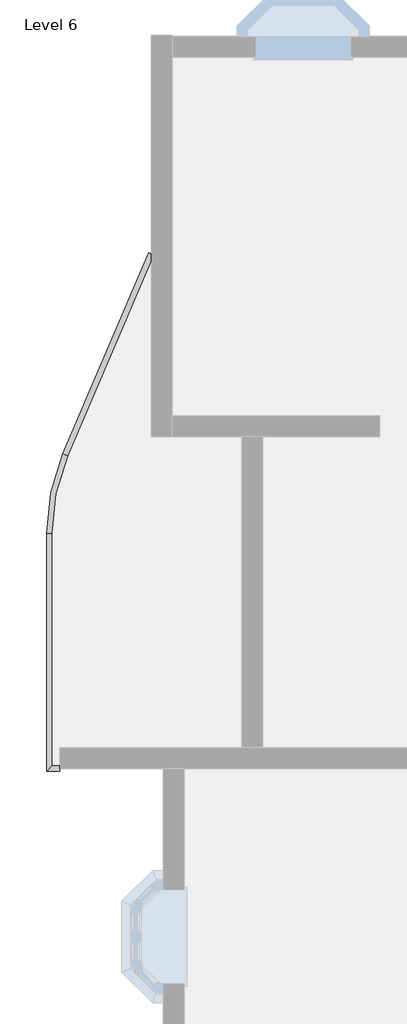
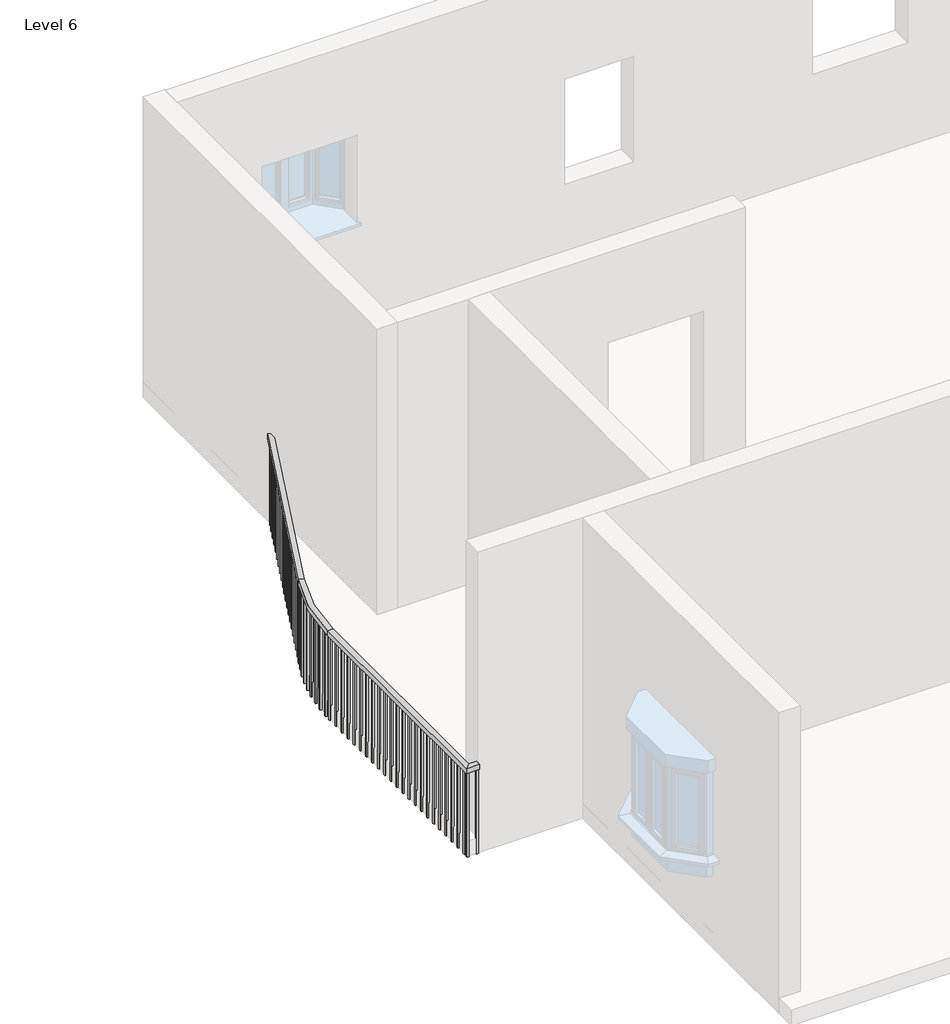
# One storey, part 7 of 14: 1 railing.
"""IFC4 building model written with IfcOpenShell, lengths in millimetres."""

from ifc_helpers import new_model, si_unit, frame, origin, place, context, project, spatial, polyline, circle_curve, outline, extrude, element, save
from ifc_brep_helpers import plane_surface, cylinder_surface, revolved_surface, advanced_brep

model = new_model("IFC4")

# Units and contexts
model_context = context("Model", 3, world=origin())
ifc_project = project(units=[si_unit("LENGTHUNIT", "METRE", prefix="MILLI")], contexts=[model_context])

# Site, building, storey
site = spatial("IfcSite", under=ifc_project)
building = spatial("IfcBuilding", under=site)
storey = spatial("IfcBuildingStorey", under=building, Name="Level 6", Elevation=15240.0)

# Railing
placement = place(None, origin())
element("IfcRailing", 1, ObjectType="Handrail - Rectangular", at=placement, inside=storey, context=model_context, shape_type="SolidModel", body=[
    advanced_brep(
    [(-12381.4379579, -2441.2590879, 16154.4), (-12381.4379579, -2441.2590879, 16103.6), (-12428.1364721, -2421.2618688, 16103.6), (-12428.1364721, -2421.2618688, 16154.4), (-13216.1814979, -4390.5942894, 16154.4), (-13216.1814979, -4390.5942894, 16103.6), (-13262.8800121, -4370.5970703, 16103.6), (-13262.8800121, -4370.5970703, 16154.4), (-13369.987215, -5140.4900045, 16103.6), (-13369.987215, -5140.4900045, 16154.4), (-13420.787215, -5140.4900045, 16103.6), (-13420.787215, -5140.4900045, 16154.4), (-13369.987215, -7396.5416506, 16154.4), (-13369.987215, -7396.5416506, 16103.6), (-13420.787215, -7447.3416506, 16103.6), (-13420.787215, -7447.3416506, 16154.4), (-13293.787215, -7396.5416506, 16154.4), (-13293.787215, -7447.3416506, 16154.4), (-13293.787215, -7447.3416506, 16103.6), (-13293.787215, -7396.5416506, 16103.6)],
    [
        (0, 1),
        (1, 2),
        (2, 3),
        (3, 0),
        (0, 4),
        (4, 5),
        (5, 1),
        (5, 6),
        (6, 2),
        (6, 7),
        (7, 3),
        (7, 4),
        (8, 5, circle_curve(frame((-11464.987215, -5140.4900045, 16103.6), z_axis=(0.0, 0.0, -1.0), x_axis=(-0.9192620907623801, 0.39364604467361003, 0.0)), 1905.0)),
        (4, 9, circle_curve(frame((-11464.987215, -5140.4900045, 16154.4), z_axis=(0.0, 0.0, 1.0), x_axis=(-0.9192620907623801, 0.39364604467361003, 0.0)), 1905.0)),
        (9, 8),
        (10, 6, circle_curve(frame((-11464.987215, -5140.4900045, 16103.6), z_axis=(0.0, 0.0, -1.0), x_axis=(-0.9192620907623801, 0.39364604467361003, 0.0)), 1955.8)),
        (8, 10),
        (11, 7, circle_curve(frame((-11464.987215, -5140.4900045, 16154.4), z_axis=(0.0, 0.0, -1.0), x_axis=(-0.9192620907623801, 0.39364604467361003, 0.0)), 1955.8)),
        (10, 11),
        (11, 9),
        (9, 12),
        (12, 13),
        (13, 8),
        (13, 14),
        (14, 10),
        (14, 15),
        (15, 11),
        (15, 12),
        (16, 17),
        (17, 18),
        (18, 19),
        (19, 16),
        (12, 16),
        (19, 13),
        (18, 14),
        (17, 15),
    ],
    [
        plane_surface(frame((-12404.787215, -2431.2604783, 16154.4), z_axis=(0.39364604467361003, 0.9192620907623801, 0.0), x_axis=(0.9192620907623801, -0.39364604467361003, 0.0))),
        plane_surface(frame((-12381.4379579, -2441.2590879, 16154.4), z_axis=(0.91926209076238, -0.39364604467361014, 0.0), x_axis=(-0.39364604467361014, -0.91926209076238, 0.0))),
        plane_surface(frame((-12381.4379579, -2441.2590879, 16103.6), z_axis=(0.0, 0.0, -1.0), x_axis=(-0.39364604467361014, -0.91926209076238, 0.0))),
        plane_surface(frame((-12428.1364721, -2421.2618688, 16103.6), z_axis=(-0.91926209076238, 0.39364604467361014, 0.0), x_axis=(-0.39364604467361014, -0.91926209076238, 0.0))),
        plane_surface(frame((-12428.1364721, -2421.2618688, 16154.4), z_axis=(0.0, 0.0, 1.0), x_axis=(-0.39364604467361014, -0.91926209076238, 0.0))),
        revolved_surface(polyline([(-13216.181497902333, -4390.594289396773, 16154.4), (-13216.181497902333, -4390.594289396773, 16103.6)]), (-11464.987215, -5140.4900045, 16154.4), (0.0, 0.0, 1.0)),
        plane_surface(frame((-11464.987215, -5140.4900045, 16103.6), z_axis=(0.0, 0.0, -1.0000000000000002), x_axis=(-0.9192620907623801, 0.39364604467361003, 0.0))),
        cylinder_surface(frame((-11464.987215, -5140.4900045, 16154.4), z_axis=(0.0, 0.0, 1.0), x_axis=(-0.9192620907623801, 0.39364604467361003, 0.0)), 1955.8),
        plane_surface(frame((-11464.987215, -5140.4900045, 16154.4), z_axis=(0.0, 0.0, 1.0000000000000002), x_axis=(-0.9192620907623801, 0.39364604467361003, 0.0))),
        plane_surface(frame((-13369.987215, -5140.4900045, 16154.4), z_axis=(1.0, 0.0, 0.0), x_axis=(0.0, -1.0, 0.0))),
        plane_surface(frame((-13369.987215, -5140.4900045, 16103.6), z_axis=(0.0, 0.0, -1.0), x_axis=(0.0, -1.0, 0.0))),
        plane_surface(frame((-13420.787215, -5140.4900045, 16103.6), z_axis=(-1.0, 0.0, 0.0), x_axis=(0.0, -1.0, 0.0))),
        plane_surface(frame((-13420.787215, -5140.4900045, 16154.4), z_axis=(0.0, 0.0, 1.0), x_axis=(0.0, -1.0, 0.0))),
        plane_surface(frame((-13293.787215, -7421.9416506, 16154.4), z_axis=(1.0, 0.0, 0.0), x_axis=(0.0, 1.0, 0.0))),
        plane_surface(frame((-13369.987215, -7396.5416506, 16154.4), z_axis=(0.0, 1.0, 0.0), x_axis=(1.0, 0.0, 0.0))),
        plane_surface(frame((-13369.987215, -7396.5416506, 16103.6), z_axis=(0.0, 0.0, -1.0), x_axis=(1.0, 0.0, 0.0))),
        plane_surface(frame((-13420.787215, -7447.3416506, 16103.6), z_axis=(0.0, -1.0, 0.0), x_axis=(1.0, 0.0, 0.0))),
        plane_surface(frame((-13420.787215, -7447.3416506, 16154.4), z_axis=(0.0, 0.0, 1.0), x_axis=(1.0, 0.0, 0.0))),
    ],
    [
        (0, [[1, 2, 3, 4]]),
        (1, [[-1, 5, 6, 7]]),
        (2, [[-2, -7, 8, 9]]),
        (3, [[-3, -9, 10, 11]]),
        (4, [[-4, -11, 12, -5]]),
        (5, [[13, -6, 14, 15]]),
        (6, [[16, -8, -13, 17]]),
        (7, [[18, -10, -16, 19]]),
        (8, [[-14, -12, -18, 20]]),
        (9, [[-15, 21, 22, 23]]),
        (10, [[-17, -23, 24, 25]]),
        (11, [[-19, -25, 26, 27]]),
        (12, [[-20, -27, 28, -21]]),
        (13, [[29, 30, 31, 32]]),
        (14, [[-22, 33, -32, 34]]),
        (15, [[-24, -34, -31, 35]]),
        (16, [[-26, -35, -30, 36]]),
        (17, [[-28, -36, -29, -33]]),
    ],
),
    extrude(outline(polyline([(-13404.912215, -7366.1650045), (-13385.862215, -7366.1650045), (-13385.862215, -7385.2150045), (-13404.912215, -7385.2150045), (-13404.912215, -7366.1650045)])), frame((0.0, 0.0, 15240.0), z_axis=(0.0, 0.0, 1.0), x_axis=(1.0, 0.0, 0.0)), (0.0, 0.0, 1.0), 863.6),
    extrude(outline(polyline([(-13404.912215, -7264.5650045), (-13385.862215, -7264.5650045), (-13385.862215, -7283.6150045), (-13404.912215, -7283.6150045), (-13404.912215, -7264.5650045)])), frame((0.0, 0.0, 15240.0), z_axis=(0.0, 0.0, 1.0), x_axis=(1.0, 0.0, 0.0)), (0.0, 0.0, 1.0), 863.6),
    extrude(outline(polyline([(-13404.912215, -7162.9650045), (-13385.862215, -7162.9650045), (-13385.862215, -7182.0150045), (-13404.912215, -7182.0150045), (-13404.912215, -7162.9650045)])), frame((0.0, 0.0, 15240.0), z_axis=(0.0, 0.0, 1.0), x_axis=(1.0, 0.0, 0.0)), (0.0, 0.0, 1.0), 863.6),
    extrude(outline(polyline([(-13404.912215, -7061.3650045), (-13385.862215, -7061.3650045), (-13385.862215, -7080.4150045), (-13404.912215, -7080.4150045), (-13404.912215, -7061.3650045)])), frame((0.0, 0.0, 15240.0), z_axis=(0.0, 0.0, 1.0), x_axis=(1.0, 0.0, 0.0)), (0.0, 0.0, 1.0), 863.6),
    extrude(outline(polyline([(-13404.912215, -6959.7650045), (-13385.862215, -6959.7650045), (-13385.862215, -6978.8150045), (-13404.912215, -6978.8150045), (-13404.912215, -6959.7650045)])), frame((0.0, 0.0, 15240.0), z_axis=(0.0, 0.0, 1.0), x_axis=(1.0, 0.0, 0.0)), (0.0, 0.0, 1.0), 863.6),
    extrude(outline(polyline([(-13404.912215, -6858.1650045), (-13385.862215, -6858.1650045), (-13385.862215, -6877.2150045), (-13404.912215, -6877.2150045), (-13404.912215, -6858.1650045)])), frame((0.0, 0.0, 15240.0), z_axis=(0.0, 0.0, 1.0), x_axis=(1.0, 0.0, 0.0)), (0.0, 0.0, 1.0), 863.6),
    extrude(outline(polyline([(-13404.912215, -6756.5650045), (-13385.862215, -6756.5650045), (-13385.862215, -6775.6150045), (-13404.912215, -6775.6150045), (-13404.912215, -6756.5650045)])), frame((0.0, 0.0, 15240.0), z_axis=(0.0, 0.0, 1.0), x_axis=(1.0, 0.0, 0.0)), (0.0, 0.0, 1.0), 863.6),
    extrude(outline(polyline([(-13404.912215, -6654.9650045), (-13385.862215, -6654.9650045), (-13385.862215, -6674.0150045), (-13404.912215, -6674.0150045), (-13404.912215, -6654.9650045)])), frame((0.0, 0.0, 15240.0), z_axis=(0.0, 0.0, 1.0), x_axis=(1.0, 0.0, 0.0)), (0.0, 0.0, 1.0), 863.6),
    extrude(outline(polyline([(-13404.912215, -6553.3650045), (-13385.862215, -6553.3650045), (-13385.862215, -6572.4150045), (-13404.912215, -6572.4150045), (-13404.912215, -6553.3650045)])), frame((0.0, 0.0, 15240.0), z_axis=(0.0, 0.0, 1.0), x_axis=(1.0, 0.0, 0.0)), (0.0, 0.0, 1.0), 863.6),
    extrude(outline(polyline([(-13404.912215, -6451.7650045), (-13385.862215, -6451.7650045), (-13385.862215, -6470.8150045), (-13404.912215, -6470.8150045), (-13404.912215, -6451.7650045)])), frame((0.0, 0.0, 15240.0), z_axis=(0.0, 0.0, 1.0), x_axis=(1.0, 0.0, 0.0)), (0.0, 0.0, 1.0), 863.6),
    extrude(outline(polyline([(-13404.912215, -6350.1650045), (-13385.862215, -6350.1650045), (-13385.862215, -6369.2150045), (-13404.912215, -6369.2150045), (-13404.912215, -6350.1650045)])), frame((0.0, 0.0, 15240.0), z_axis=(0.0, 0.0, 1.0), x_axis=(1.0, 0.0, 0.0)), (0.0, 0.0, 1.0), 863.6),
    extrude(outline(polyline([(-13404.912215, -6248.5650045), (-13385.862215, -6248.5650045), (-13385.862215, -6267.6150045), (-13404.912215, -6267.6150045), (-13404.912215, -6248.5650045)])), frame((0.0, 0.0, 15240.0), z_axis=(0.0, 0.0, 1.0), x_axis=(1.0, 0.0, 0.0)), (0.0, 0.0, 1.0), 863.6),
    extrude(outline(polyline([(-13404.912215, -6146.9650045), (-13385.862215, -6146.9650045), (-13385.862215, -6166.0150045), (-13404.912215, -6166.0150045), (-13404.912215, -6146.9650045)])), frame((0.0, 0.0, 15240.0), z_axis=(0.0, 0.0, 1.0), x_axis=(1.0, 0.0, 0.0)), (0.0, 0.0, 1.0), 863.6),
    extrude(outline(polyline([(-13404.912215, -6045.3650045), (-13385.862215, -6045.3650045), (-13385.862215, -6064.4150045), (-13404.912215, -6064.4150045), (-13404.912215, -6045.3650045)])), frame((0.0, 0.0, 15240.0), z_axis=(0.0, 0.0, 1.0), x_axis=(1.0, 0.0, 0.0)), (0.0, 0.0, 1.0), 863.6),
    extrude(outline(polyline([(-13404.912215, -5943.7650045), (-13385.862215, -5943.7650045), (-13385.862215, -5962.8150045), (-13404.912215, -5962.8150045), (-13404.912215, -5943.7650045)])), frame((0.0, 0.0, 15240.0), z_axis=(0.0, 0.0, 1.0), x_axis=(1.0, 0.0, 0.0)), (0.0, 0.0, 1.0), 863.6),
    extrude(outline(polyline([(-13404.912215, -5842.1650045), (-13385.862215, -5842.1650045), (-13385.862215, -5861.2150045), (-13404.912215, -5861.2150045), (-13404.912215, -5842.1650045)])), frame((0.0, 0.0, 15240.0), z_axis=(0.0, 0.0, 1.0), x_axis=(1.0, 0.0, 0.0)), (0.0, 0.0, 1.0), 863.6),
    extrude(outline(polyline([(-13404.912215, -5740.5650045), (-13385.862215, -5740.5650045), (-13385.862215, -5759.6150045), (-13404.912215, -5759.6150045), (-13404.912215, -5740.5650045)])), frame((0.0, 0.0, 15240.0), z_axis=(0.0, 0.0, 1.0), x_axis=(1.0, 0.0, 0.0)), (0.0, 0.0, 1.0), 863.6),
    extrude(outline(polyline([(-13404.912215, -5638.9650045), (-13385.862215, -5638.9650045), (-13385.862215, -5658.0150045), (-13404.912215, -5658.0150045), (-13404.912215, -5638.9650045)])), frame((0.0, 0.0, 15240.0), z_axis=(0.0, 0.0, 1.0), x_axis=(1.0, 0.0, 0.0)), (0.0, 0.0, 1.0), 863.6),
    extrude(outline(polyline([(-13404.912215, -5537.3650045), (-13385.862215, -5537.3650045), (-13385.862215, -5556.4150045), (-13404.912215, -5556.4150045), (-13404.912215, -5537.3650045)])), frame((0.0, 0.0, 15240.0), z_axis=(0.0, 0.0, 1.0), x_axis=(1.0, 0.0, 0.0)), (0.0, 0.0, 1.0), 863.6),
    extrude(outline(polyline([(-13404.912215, -5435.7650045), (-13385.862215, -5435.7650045), (-13385.862215, -5454.8150045), (-13404.912215, -5454.8150045), (-13404.912215, -5435.7650045)])), frame((0.0, 0.0, 15240.0), z_axis=(0.0, 0.0, 1.0), x_axis=(1.0, 0.0, 0.0)), (0.0, 0.0, 1.0), 863.6),
    extrude(outline(polyline([(-13404.912215, -5334.1650045), (-13385.862215, -5334.1650045), (-13385.862215, -5353.2150045), (-13404.912215, -5353.2150045), (-13404.912215, -5334.1650045)])), frame((0.0, 0.0, 15240.0), z_axis=(0.0, 0.0, 1.0), x_axis=(1.0, 0.0, 0.0)), (0.0, 0.0, 1.0), 863.6),
    extrude(outline(polyline([(-13404.912215, -5232.5650045), (-13385.862215, -5232.5650045), (-13385.862215, -5251.6150045), (-13404.912215, -5251.6150045), (-13404.912215, -5232.5650045)])), frame((0.0, 0.0, 15240.0), z_axis=(0.0, 0.0, 1.0), x_axis=(1.0, 0.0, 0.0)), (0.0, 0.0, 1.0), 863.6),
    extrude(outline(polyline([(-13403.2986616, -5060.8127369), (-13384.2611239, -5061.5016911), (-13384.9500781, -5080.5392288), (-13403.9876158, -5079.8502746), (-13403.2986616, -5060.8127369)])), frame((0.0, 0.0, 15240.0), z_axis=(0.0, 0.0, 1.0), x_axis=(1.0, 0.0, 0.0)), (0.0, 0.0, 1.0), 863.6),
    extrude(outline(polyline([(-13396.4230348, -4958.9537683), (-13377.4481028, -4960.6432816), (-13379.1376161, -4979.6182136), (-13398.1125481, -4977.9287003), (-13396.4230348, -4958.9537683)])), frame((0.0, 0.0, 15240.0), z_axis=(0.0, 0.0, 1.0), x_axis=(1.0, 0.0, 0.0)), (0.0, 0.0, 1.0), 863.6),
    extrude(outline(polyline([(-13384.1984052, -4857.5975541), (-13365.3386289, -4860.2829475), (-13368.0240223, -4879.1427238), (-13386.8837986, -4876.4573304), (-13384.1984052, -4857.5975541)])), frame((0.0, 0.0, 15240.0), z_axis=(0.0, 0.0, 1.0), x_axis=(1.0, 0.0, 0.0)), (0.0, 0.0, 1.0), 863.6),
    extrude(outline(polyline([(-13366.6586282, -4757.0247946), (-13347.9662387, -4760.698631), (-13351.6400752, -4779.3910205), (-13370.3324647, -4775.7171841), (-13366.6586282, -4757.0247946)])), frame((0.0, 0.0, 15240.0), z_axis=(0.0, 0.0, 1.0), x_axis=(1.0, 0.0, 0.0)), (0.0, 0.0, 1.0), 863.6),
    extrude(outline(polyline([(-13343.8522793, -4657.5140204), (-13325.3790441, -4662.1661254), (-13330.0311492, -4680.6393606), (-13348.5043844, -4675.9872556), (-13343.8522793, -4657.5140204)])), frame((0.0, 0.0, 15240.0), z_axis=(0.0, 0.0, 1.0), x_axis=(1.0, 0.0, 0.0)), (0.0, 0.0, 1.0), 863.6),
    extrude(outline(polyline([(-13315.8425193, -4559.340821), (-13297.6395991, -4564.9583109), (-13303.257089, -4583.1612312), (-13321.4600093, -4577.5437413), (-13315.8425193, -4559.340821)])), frame((0.0, 0.0, 15240.0), z_axis=(0.0, 0.0, 1.0), x_axis=(1.0, 0.0, 0.0)), (0.0, 0.0, 1.0), 863.6),
    extrude(outline(polyline([(-13282.7069198, -4462.7770815), (-13264.8247264, -4469.344399), (-13271.3920438, -4487.2265924), (-13289.2742372, -4480.659275), (-13282.7069198, -4462.7770815)])), frame((0.0, 0.0, 15240.0), z_axis=(0.0, 0.0, 1.0), x_axis=(1.0, 0.0, 0.0)), (0.0, 0.0, 1.0), 863.6),
    extrude(outline(polyline([(-13209.6824706, -4286.6955968), (-13192.1705278, -4294.1945539), (-13199.6694849, -4311.7064967), (-13217.1814277, -4304.2075396), (-13209.6824706, -4286.6955968)])), frame((0.0, 0.0, 15240.0), z_axis=(0.0, 0.0, 1.0), x_axis=(1.0, 0.0, 0.0)), (0.0, 0.0, 1.0), 863.6),
    extrude(outline(polyline([(-13169.6880325, -4193.2985683), (-13152.1760896, -4200.7975255), (-13159.6750468, -4218.3094683), (-13177.1869896, -4210.8105112), (-13169.6880325, -4193.2985683)])), frame((0.0, 0.0, 15240.0), z_axis=(0.0, 0.0, 1.0), x_axis=(1.0, 0.0, 0.0)), (0.0, 0.0, 1.0), 863.6),
    extrude(outline(polyline([(-13129.6935943, -4099.9015399), (-13112.1816515, -4107.4004971), (-13119.6806086, -4124.9124399), (-13137.1925515, -4117.4134827), (-13129.6935943, -4099.9015399)])), frame((0.0, 0.0, 15240.0), z_axis=(0.0, 0.0, 1.0), x_axis=(1.0, 0.0, 0.0)), (0.0, 0.0, 1.0), 863.6),
    extrude(outline(polyline([(-13089.6991562, -4006.5045115), (-13072.1872133, -4014.0034686), (-13079.6861705, -4031.5154115), (-13097.1981133, -4024.0164543), (-13089.6991562, -4006.5045115)])), frame((0.0, 0.0, 15240.0), z_axis=(0.0, 0.0, 1.0), x_axis=(1.0, 0.0, 0.0)), (0.0, 0.0, 1.0), 863.6),
    extrude(outline(polyline([(-13049.704718, -3913.1074831), (-13032.1927752, -3920.6064402), (-13039.6917324, -3938.1183831), (-13057.2036752, -3930.6194259), (-13049.704718, -3913.1074831)])), frame((0.0, 0.0, 15240.0), z_axis=(0.0, 0.0, 1.0), x_axis=(1.0, 0.0, 0.0)), (0.0, 0.0, 1.0), 863.6),
    extrude(outline(polyline([(-13009.7102799, -3819.7104546), (-12992.1983371, -3827.2094118), (-12999.6972942, -3844.7213546), (-13017.209237, -3837.2223975), (-13009.7102799, -3819.7104546)])), frame((0.0, 0.0, 15240.0), z_axis=(0.0, 0.0, 1.0), x_axis=(1.0, 0.0, 0.0)), (0.0, 0.0, 1.0), 863.6),
    extrude(outline(polyline([(-12969.7158418, -3726.3134262), (-12952.2038989, -3733.8123834), (-12959.7028561, -3751.3243262), (-12977.2147989, -3743.8253691), (-12969.7158418, -3726.3134262)])), frame((0.0, 0.0, 15240.0), z_axis=(0.0, 0.0, 1.0), x_axis=(1.0, 0.0, 0.0)), (0.0, 0.0, 1.0), 863.6),
    extrude(outline(polyline([(-12929.7214036, -3632.9163978), (-12912.2094608, -3640.415355), (-12919.7084179, -3657.9272978), (-12937.2203608, -3650.4283406), (-12929.7214036, -3632.9163978)])), frame((0.0, 0.0, 15240.0), z_axis=(0.0, 0.0, 1.0), x_axis=(1.0, 0.0, 0.0)), (0.0, 0.0, 1.0), 863.6),
    extrude(outline(polyline([(-12889.7269655, -3539.5193694), (-12872.2150227, -3547.0183265), (-12879.7139798, -3564.5302694), (-12897.2259226, -3557.0313122), (-12889.7269655, -3539.5193694)])), frame((0.0, 0.0, 15240.0), z_axis=(0.0, 0.0, 1.0), x_axis=(1.0, 0.0, 0.0)), (0.0, 0.0, 1.0), 863.6),
    extrude(outline(polyline([(-12849.7325273, -3446.122341), (-12832.2205845, -3453.6212981), (-12839.7195417, -3471.1332409), (-12857.2314845, -3463.6342838), (-12849.7325273, -3446.122341)])), frame((0.0, 0.0, 15240.0), z_axis=(0.0, 0.0, 1.0), x_axis=(1.0, 0.0, 0.0)), (0.0, 0.0, 1.0), 863.6),
    extrude(outline(polyline([(-12809.7380892, -3352.7253125), (-12792.2261464, -3360.2242697), (-12799.7251035, -3377.7362125), (-12817.2370464, -3370.2372554), (-12809.7380892, -3352.7253125)])), frame((0.0, 0.0, 15240.0), z_axis=(0.0, 0.0, 1.0), x_axis=(1.0, 0.0, 0.0)), (0.0, 0.0, 1.0), 863.6),
    extrude(outline(polyline([(-12769.7436511, -3259.3282841), (-12752.2317082, -3266.8272413), (-12759.7306654, -3284.3391841), (-12777.2426082, -3276.8402269), (-12769.7436511, -3259.3282841)])), frame((0.0, 0.0, 15240.0), z_axis=(0.0, 0.0, 1.0), x_axis=(1.0, 0.0, 0.0)), (0.0, 0.0, 1.0), 863.6),
    extrude(outline(polyline([(-12729.7492129, -3165.9312557), (-12712.2372701, -3173.4302129), (-12719.7362272, -3190.9421557), (-12737.2481701, -3183.4431985), (-12729.7492129, -3165.9312557)])), frame((0.0, 0.0, 15240.0), z_axis=(0.0, 0.0, 1.0), x_axis=(1.0, 0.0, 0.0)), (0.0, 0.0, 1.0), 863.6),
    extrude(outline(polyline([(-12689.7547748, -3072.5342273), (-12672.242832, -3080.0331844), (-12679.7417891, -3097.5451273), (-12697.2537319, -3090.0461701), (-12689.7547748, -3072.5342273)])), frame((0.0, 0.0, 15240.0), z_axis=(0.0, 0.0, 1.0), x_axis=(1.0, 0.0, 0.0)), (0.0, 0.0, 1.0), 863.6),
    extrude(outline(polyline([(-12649.7603366, -2979.1371989), (-12632.2483938, -2986.636156), (-12639.747351, -3004.1480988), (-12657.2592938, -2996.6491417), (-12649.7603366, -2979.1371989)])), frame((0.0, 0.0, 15240.0), z_axis=(0.0, 0.0, 1.0), x_axis=(1.0, 0.0, 0.0)), (0.0, 0.0, 1.0), 863.6),
    extrude(outline(polyline([(-12609.7658985, -2885.7401704), (-12592.2539557, -2893.2391276), (-12599.7529128, -2910.7510704), (-12617.2648557, -2903.2521133), (-12609.7658985, -2885.7401704)])), frame((0.0, 0.0, 15240.0), z_axis=(0.0, 0.0, 1.0), x_axis=(1.0, 0.0, 0.0)), (0.0, 0.0, 1.0), 863.6),
    extrude(outline(polyline([(-12569.7714604, -2792.343142), (-12552.2595175, -2799.8420992), (-12559.7584747, -2817.354042), (-12577.2704175, -2809.8550848), (-12569.7714604, -2792.343142)])), frame((0.0, 0.0, 15240.0), z_axis=(0.0, 0.0, 1.0), x_axis=(1.0, 0.0, 0.0)), (0.0, 0.0, 1.0), 863.6),
    extrude(outline(polyline([(-12529.7770222, -2698.9461136), (-12512.2650794, -2706.4450707), (-12519.7640366, -2723.9570136), (-12537.2759794, -2716.4580564), (-12529.7770222, -2698.9461136)])), frame((0.0, 0.0, 15240.0), z_axis=(0.0, 0.0, 1.0), x_axis=(1.0, 0.0, 0.0)), (0.0, 0.0, 1.0), 863.6),
    extrude(outline(polyline([(-12489.7825841, -2605.5490852), (-12472.2706413, -2613.0480423), (-12479.7695984, -2630.5599852), (-12497.2815412, -2623.061028), (-12489.7825841, -2605.5490852)])), frame((0.0, 0.0, 15240.0), z_axis=(0.0, 0.0, 1.0), x_axis=(1.0, 0.0, 0.0)), (0.0, 0.0, 1.0), 863.6),
    extrude(outline(polyline([(-12449.788146, -2512.1520567), (-12432.2762031, -2519.6510139), (-12439.7751603, -2537.1629567), (-12457.2871031, -2529.6639996), (-12449.788146, -2512.1520567)])), frame((0.0, 0.0, 15240.0), z_axis=(0.0, 0.0, 1.0), x_axis=(1.0, 0.0, 0.0)), (0.0, 0.0, 1.0), 863.6),
    extrude(outline(polyline([(-13404.912215, -7412.4166506), (-13385.862215, -7412.4166506), (-13385.862215, -7431.4666506), (-13404.912215, -7431.4666506), (-13404.912215, -7412.4166506)])), frame((0.0, 0.0, 15240.0), z_axis=(0.0, 0.0, 1.0), x_axis=(1.0, 0.0, 0.0)), (0.0, 0.0, 1.0), 863.6),
    extrude(outline(polyline([(-13404.912215, -5130.9650045), (-13385.862215, -5130.9650045), (-13385.862215, -5150.0150045), (-13404.912215, -5150.0150045), (-13404.912215, -5130.9650045)])), frame((0.0, 0.0, 15240.0), z_axis=(0.0, 0.0, 1.0), x_axis=(1.0, 0.0, 0.0)), (0.0, 0.0, 1.0), 863.6),
    extrude(outline(polyline([(-13244.5372478, -4368.0902299), (-13227.025305, -4375.589187), (-13234.5242621, -4393.1011299), (-13252.036205, -4385.6021727), (-13244.5372478, -4368.0902299)])), frame((0.0, 0.0, 15240.0), z_axis=(0.0, 0.0, 1.0), x_axis=(1.0, 0.0, 0.0)), (0.0, 0.0, 1.0), 863.6),
    extrude(outline(polyline([(-13312.837215, -7431.4666506), (-13312.837215, -7412.4166506), (-13293.787215, -7412.4166506), (-13293.787215, -7431.4666506), (-13312.837215, -7431.4666506)])), frame((0.0, 0.0, 15240.0), z_axis=(0.0, 0.0, 1.0), x_axis=(1.0, 0.0, 0.0)), (0.0, 0.0, 1.0), 863.6),
    extrude(outline(polyline([(-12413.5431864, -2427.5109997), (-12396.0312436, -2435.0099569), (-12403.5302007, -2452.5218997), (-12421.0421435, -2445.0229426), (-12413.5431864, -2427.5109997)])), frame((0.0, 0.0, 15240.0), z_axis=(0.0, 0.0, 1.0), x_axis=(1.0, 0.0, 0.0)), (0.0, 0.0, 1.0), 863.6),
])

save(model, "model.ifc")

# Revit data of these elements
# Type "Handrail - Rectangular"
#   Assembly Code = "C2010400"
#   built-in parameter 1008612 = 0.0416667 (stored number, unit not read)
#   built-in parameter 1008611 = 0.0416667 (stored number, unit not read)
#   built-in parameter 1008609 = 0.333333 (stored number, unit not read)
#   built-in parameter 1008604 = 0.166667 (stored number, unit not read)
#   built-in parameter 1008603 = 0.166667 (stored number, unit not read)
#   Railing Height = 3' - 0"
#   built-in parameter 1008630 = 2
#   built-in parameter 1008610 = 2
#   built-in parameter 1008618 = Baluster - Square : 3/4"
# Element 1 (IfcRailing, "Handrail - Rectangular")
#   Phase Created = New Construction
